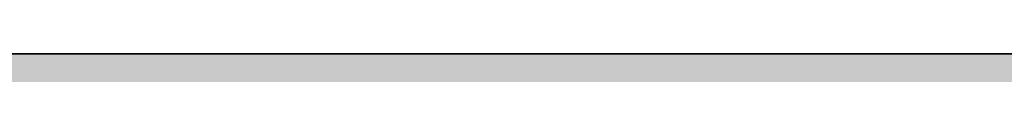
# Model space of a CAD drawing. Units: inches. Extents: x 2091 to 2899, y 967 to 2217.
# Tile 53 of 256: x 2212.15117 to 2212.16216, y 1099.91883 to 1099.91906. Entities that reach past the tile are written whole.
import ezdxf

# ---------------------------------------------------------------- set-up
doc = ezdxf.new("R2010")
doc.units = ezdxf.units.IN
doc.layers.add('A-WALL-PATT', color=141, linetype='Continuous', lineweight=13, true_color=0xadddf7)
doc.layers.add('L-SITE-WALL', color=7, linetype='Continuous', lineweight=35)

msp = doc.modelspace()

# ---------------------------------------------------------------- hatches: boundary and pattern name
at = {"layer": 'A-WALL-PATT'}
h = msp.add_hatch(color=256, dxfattribs=at)
h.dxf.hatch_style = 1
h.paths.add_polyline_path([(2212.143603, 1941.419059), (2387.643603, 1941.419059), (2387.643603, 1824.419059), (2392.143603, 1824.419059), (2392.143603, 1941.419059), (2609.643603, 1941.419059), (2609.643603, 1825.919059), (2614.143603, 1825.919059), (2614.143603, 1941.419059), (2794.143603, 1941.419059), (2794.143603, 1928.762166), (2803.143603, 1928.762166), (2803.143603, 2050.919059), (2203.143603, 2050.919059), (2203.143603, 1900.757859), (2212.143603, 1900.757859)])
h.paths.add_polyline_path([(2212.143603, 1945.919059), (2212.143603, 2041.919059), (2794.143603, 2041.919059), (2794.143603, 1945.919059), (2402.248245, 1945.919059), (2401.102434, 1945.775832), (2398.702434, 1945.775832)], flags=16)
h.paths.add_polyline_path([(2230.229861, 1948.062793), (2227.349861, 1949.502793), (2225.909861, 1951.902793), (2223.989861, 1952.862793), (2223.029861, 1955.262793), (2222.069861, 1959.582793), (2222.069861, 1963.422793), (2223.029861, 1965.662793), (2223.989861, 1965.342793), (2225.58591, 1963.860747), (2226.911533, 1964.957259), (2226.948861, 1965.938793), (2227.778319, 1966.952143), (2228.199916, 1968.878704), (2230.709861, 1964.862793), (2233.589861, 1966.302793), (2233.607309, 1966.331873), (2233.772659, 1964.938205), (2234.633802, 1963.676473), (2235.029861, 1963.902793), (2236.282035, 1965.572358), (2235.989861, 1962.942793), (2237.954512, 1957.540002), (2238.389861, 1957.902793), (2239.215861, 1960.305793), (2238.654565, 1966.38496), (2238.692792, 1966.438069), (2238.840578, 1967.499707), (2238.780291, 1967.687486), (2238.880538, 1967.786763), (2238.666861, 1966.251793), (2239.215861, 1960.305793), (2238.389861, 1957.902793), (2236.949861, 1956.702793), (2234.549861, 1949.982793)], flags=0)
h.paths.add_polyline_path([(2278.011974, 1948.062793), (2276.496427, 1947.873349), (2275.849833, 1947.688608), (2274.651974, 1947.102793)], flags=0)
h.paths.add_polyline_path([(2269.851974, 1955.742793), (2268.276176, 1956.629329), (2270.867302, 1956.348398), (2269.371974, 1958.142793), (2268.714964, 1959.192325), (2270.569833, 1958.728608), (2268.580725, 1961.906087), (2270.811974, 1960.891883), (2270.811974, 1963.422793), (2271.393315, 1964.779256), (2270.291762, 1966.156196), (2271.771974, 1965.662793), (2272.141387, 1966.524757), (2273.929833, 1965.928608), (2275.630385, 1968.054299), (2276.331938, 1966.72186), (2276.520431, 1966.952143), (2276.942029, 1968.878704), (2277.734293, 1967.611082), (2278.139888, 1969.46452), (2279.659124, 1967.033742), (2280.411974, 1966.782793), (2280.949302, 1967.588785), (2281.609833, 1967.368608), (2282.133266, 1968.153758), (2282.349235, 1966.333445), (2282.349849, 1966.332585), (2283.40755, 1968.09542), (2283.712631, 1965.52402), (2284.320221, 1964.633789), (2284.511809, 1964.889239), (2284.234974, 1965.704793), (2284.500472, 1967.318958), (2284.907944, 1965.41742), (2285.396313, 1966.068579), (2285.432833, 1966.290608), (2285.473338, 1966.171279), (2286.353919, 1967.345387), (2286.222007, 1966.158173), (2287.663492, 1968.080154), (2287.713974, 1968.442793), (2288.481599, 1969.016679), (2288.573993, 1968.728897), (2288.917461, 1969.06904), (2288.606833, 1966.837608), (2288.928726, 1963.35131), (2288.934974, 1963.356793), (2288.929731, 1963.340422), (2289.015281, 1962.413869), (2290.111223, 1963.875126), (2290.132833, 1963.942608), (2290.217672, 1964.017058), (2290.111223, 1963.875126), (2289.155833, 1960.891608), (2288.594036, 1959.257227), (2288.571974, 1959.102793), (2289.531974, 1960.542793), (2290.011974, 1962.462793), (2290.19184, 1962.642659), (2289.769833, 1959.688608), (2286.889833, 1957.288608), (2284.489833, 1950.568608), (2283.314658, 1950.046308), (2283.291974, 1949.982793), (2280.290059, 1948.648608), (2281.129833, 1948.648608), (2282.569833, 1948.168608), (2283.204726, 1948.062793), (2278.971974, 1948.062793), (2276.091974, 1949.502793), (2274.651974, 1951.902793), (2272.731974, 1952.862793)], flags=0)
h.paths.add_polyline_path([(2271.158868, 1958.021765), (2272.969833, 1955.848608), (2272.009833, 1960.168608), (2272.009833, 1964.008608), (2272.624426, 1965.442658), (2274.328023, 1963.860747), (2275.653646, 1964.957259), (2275.637743, 1964.53909), (2277.412231, 1966.006888), (2277.032974, 1965.156793), (2276.829924, 1964.975597), (2276.766012, 1963.295014), (2277.449635, 1962.66022), (2279.451974, 1964.862793), (2282.331974, 1966.302793), (2283.529833, 1966.888608), (2283.294512, 1966.770948), (2283.912993, 1963.8847), (2284.899249, 1964.448275), (2284.731974, 1962.942793), (2286.696625, 1957.540002), (2287.131974, 1957.902793), (2287.541913, 1959.095388), (2287.779395, 1958.442311), (2285.682738, 1956.695097), (2285.876503, 1959.795336), (2284.731974, 1962.942793), (2284.899249, 1964.448275), (2283.912993, 1963.8847), (2284.223833, 1962.434116), (2283.424365, 1963.605484), (2281.609833, 1962.568608), (2281.129833, 1960.168608), (2282.089833, 1956.328608), (2283.049833, 1952.968608), (2282.569833, 1950.568608), (2280.169833, 1948.648608), (2279.883316, 1948.791867), (2278.971974, 1948.062793), (2278.971974, 1949.022793), (2278.672313, 1949.397368), (2277.289833, 1950.088608), (2275.849833, 1952.488608), (2273.929833, 1953.448608), (2272.489833, 1954.888608), (2271.921647, 1954.888608), (2271.771974, 1955.262793)], flags=0)
h.paths.add_polyline_path([(2311.994146, 1955.742793), (2312.062717, 1955.674221), (2312.0551, 1955.7085)], flags=0)
h.paths.add_polyline_path([(2331.956146, 1963.951793), (2333.396146, 1965.391793), (2331.077146, 1963.356793), (2330.998603, 1963.111517)], flags=0)
h.paths.add_polyline_path([(2310.554146, 1954.302793), (2307.039807, 1956.279943), (2310.762903, 1955.876284), (2312.474146, 1953.822793), (2313.434146, 1951.422793), (2315.354146, 1950.462793), (2316.794146, 1948.062793), (2317.466146, 1947.726793), (2319.368691, 1947.964611), (2317.754146, 1949.982793), (2317.569531, 1950.610485), (2316.794146, 1951.902793), (2314.874146, 1952.862793), (2313.914146, 1955.262793), (2311.514146, 1958.142793), (2309.375489, 1961.559168), (2311.514146, 1960.337078), (2311.514146, 1961.982793), (2310.604672, 1963.119635), (2311.726605, 1962.47853), (2312.418332, 1964.09256), (2312.255964, 1964.29552), (2313.194146, 1963.982793), (2313.914146, 1965.662793), (2314.646778, 1965.418582), (2315.354146, 1966.302793), (2316.794146, 1967.742793), (2316.157435, 1966.946904), (2317.034111, 1965.28186), (2317.222604, 1965.512143), (2317.777048, 1968.045771), (2318.474111, 1966.72186), (2318.662604, 1966.952143), (2319.084201, 1968.878704), (2321.207049, 1965.482147), (2322.161419, 1966.913702), (2322.554146, 1966.782793), (2322.785988, 1967.130555), (2322.881646, 1966.324293), (2323.312041, 1965.72174), (2323.651289, 1965.891364), (2324.3965, 1967.133382), (2324.656945, 1964.938205), (2324.971986, 1964.476611), (2325.38728, 1967.001499), (2325.940813, 1964.418348), (2327.228929, 1966.135836), (2327.16632, 1965.572358), (2328.059139, 1966.762783), (2328.224576, 1966.247486), (2329.667971, 1967.67691), (2329.664576, 1967.687486), (2329.764823, 1967.786763), (2329.551146, 1966.251793), (2330.100146, 1960.305793), (2329.332814, 1958.07347), (2329.313065, 1957.935225), (2329.634146, 1958.202793), (2330.234146, 1959.102793), (2330.714146, 1961.022793), (2331.034146, 1961.342793), (2330.714146, 1959.102793), (2329.634146, 1958.202793), (2329.274146, 1957.662793), (2327.712112, 1956.361098), (2325.434146, 1949.982793), (2324.333769, 1949.493736), (2323.994146, 1948.542793), (2319.674146, 1946.622793), (2316.794146, 1948.062793), (2315.354146, 1950.462793), (2313.434146, 1951.422793)], flags=0)
h.paths.add_polyline_path([(2321.335684, 1947.952023), (2321.114146, 1948.062793), (2321.114146, 1949.022793), (2319.194146, 1951.422793), (2316.794146, 1959.582793), (2316.663237, 1959.582793), (2315.354146, 1958.142793), (2314.394146, 1958.142793), (2313.148303, 1958.709085), (2312.954146, 1959.582793), (2312.954146, 1960.891883), (2315.834146, 1959.582793), (2316.663237, 1959.582793), (2317.314709, 1960.299412), (2315.030195, 1962.420747), (2316.355818, 1963.517259), (2316.372337, 1963.951615), (2316.470195, 1963.860747), (2317.795818, 1964.957259), (2317.755219, 1963.889687), (2319.175146, 1965.156793), (2319.498407, 1965.881372), (2321.114146, 1965.342793), (2323.235885, 1962.372358), (2325.686349, 1963.772623), (2325.542789, 1962.480576), (2325.198783, 1963.494014), (2324.47851, 1963.082429), (2324.926005, 1960.994116), (2324.078087, 1962.236473), (2322.414791, 1961.286018), (2322.074146, 1959.582793), (2323.034146, 1955.742793), (2323.994146, 1952.382793), (2323.514146, 1949.982793), (2322.142717, 1948.88565), (2322.074146, 1948.542793)], flags=0)
h.paths.add_polyline_path([(2320.207479, 1963.337459), (2320.154146, 1963.422793), (2320.394146, 1963.542793)], flags=0)
h.paths.add_polyline_path([(2353.850527, 1965.8105), (2354.030527, 1965.7505), (2354.330527, 1966.4505), (2354.330527, 1966.9305)], flags=0)
h.paths.add_polyline_path([(2359.020582, 1969.026412), (2359.098382, 1968.901932), (2359.233527, 1969.5195), (2359.233527, 1969.9995)], flags=0)
h.paths.add_polyline_path([(2358.256694, 1966.681672), (2357.983601, 1966.348035), (2358.211267, 1966.146175), (2358.410492, 1966.389568)], flags=0)
h.paths.add_polyline_path([(2357.768473, 1966.058778), (2357.7322, 1965.104967), (2357.751047, 1965.120556), (2357.769527, 1965.6065), (2357.769527, 1966.057843)], flags=0)
h.paths.add_polyline_path([(2359.111527, 1965.3045), (2359.111527, 1964.8245), (2359.844527, 1966.4675), (2359.844527, 1966.9475)], flags=0)
h.paths.add_polyline_path([(2360.223684, 1966.621449), (2360.698527, 1969.3625), (2360.698527, 1969.8425), (2360.210527, 1967.0255), (2360.210527, 1966.6425)], flags=0)
h.paths.add_polyline_path([(2363.450527, 1967.8905), (2363.450527, 1968.3705), (2362.490527, 1966.9305), (2362.656045, 1966.698776)], flags=0)
h.paths.add_polyline_path([(2364.475523, 1966.078826), (2365.850527, 1968.3705), (2365.850527, 1968.8505), (2364.427975, 1966.479581)], flags=0)
h.paths.add_polyline_path([(2366.313527, 1965.8525), (2366.366709, 1965.695829), (2366.802527, 1968.3455), (2366.802527, 1968.8255)], flags=0)
h.paths.add_polyline_path([(2367.16531, 1965.803544), (2367.290527, 1966.9305), (2367.290527, 1967.4105), (2367.102701, 1965.720066)], flags=0)
h.paths.add_polyline_path([(2370.036527, 1959.9735), (2371.013527, 1963.0245), (2371.013527, 1963.5045), (2370.036527, 1960.4535)], flags=0)
h.paths.add_polyline_path([(2371.610527, 1960.2105), (2372.570527, 1961.6505), (2372.570527, 1962.1305), (2371.802527, 1960.9785)], flags=0)
h.paths.add_polyline_path([(2350.873666, 1956.005086), (2351.930527, 1955.8905), (2354.490527, 1953.3305), (2353.850527, 1954.9305), (2351.450527, 1957.8105), (2347.935527, 1963.4255), (2347.935527, 1963.9055), (2351.450527, 1958.2905), (2353.705073, 1955.585046), (2352.890527, 1959.2505), (2352.890527, 1959.7305), (2352.890527, 1961.924786), (2356.730527, 1959.7305), (2358.454471, 1961.626838), (2354.810527, 1965.0105), (2355.030855, 1965.28591), (2358.691091, 1961.88712), (2361.530527, 1965.0105), (2364.376495, 1966.433484), (2364.524394, 1965.186911), (2365.454468, 1963.824181), (2365.881073, 1964.067955), (2365.370527, 1966.4505), (2365.370527, 1966.9305), (2366.810527, 1960.2105), (2366.810527, 1959.7305), (2366.388709, 1952.981409), (2367.770527, 1956.8505), (2368.641225, 1957.576082), (2366.810527, 1962.6105), (2366.810527, 1963.0905), (2368.775179, 1957.68771), (2369.210527, 1958.0505), (2370.001592, 1960.351867), (2369.475232, 1966.052668), (2369.513458, 1966.105777), (2369.514173, 1966.110912), (2369.475232, 1966.532668), (2369.513458, 1966.585777), (2369.614635, 1967.312591), (2369.182527, 1968.6585), (2369.182527, 1969.1385), (2369.600957, 1967.835194), (2369.701204, 1967.934471), (2369.717947, 1968.054743), (2370.145176, 1968.374145), (2369.778707, 1968.011224), (2369.701204, 1967.454471), (2370.468161, 1968.214004), (2369.674936, 1967.265771), (2369.514173, 1966.110912), (2370.036527, 1960.4535), (2370.036527, 1959.9735), (2369.441756, 1958.243191), (2370.650527, 1959.2505), (2371.045821, 1962.017559), (2371.130527, 1962.1305), (2370.650527, 1958.7705), (2367.770527, 1956.3705), (2365.370527, 1949.6505), (2362.079099, 1948.187643), (2363.450527, 1947.7305), (2361.050527, 1947.7305), (2360.090527, 1947.7305), (2357.103861, 1947.357167), (2360.090527, 1948.2105), (2358.170527, 1949.1705), (2356.730527, 1951.5705), (2354.810527, 1952.5305), (2351.930527, 1955.4105)], flags=0)
h.paths.add_polyline_path([(2361.050527, 1948.6905), (2359.130527, 1951.0905), (2356.730527, 1959.2505), (2355.770527, 1959.2505), (2352.890527, 1960.559591), (2352.890527, 1961.444786), (2355.890527, 1959.7305), (2356.730527, 1959.7305), (2356.837194, 1959.367834), (2361.530527, 1964.5305), (2363.248422, 1965.389448), (2364.92531, 1963.041805), (2362.490527, 1961.6505), (2362.063861, 1959.517167), (2362.970527, 1955.8905), (2363.930527, 1952.5305), (2363.930527, 1952.0505), (2363.450527, 1949.6505), (2361.050527, 1947.7305)], flags=0)
h.paths.add_polyline_path([(2359.130527, 1951.5705), (2359.290527, 1951.3705), (2361.050527, 1954.4505), (2361.050527, 1954.9305)], flags=0)
h.paths.add_polyline_path([(2357.219527, 1966.5455), (2356.792527, 1968.8145), (2356.792527, 1969.2945), (2357.219527, 1967.0255)], flags=0)
h.paths.add_polyline_path([(2361.050527, 1954.4505), (2361.530527, 1958.7705), (2361.530527, 1959.2505), (2361.050527, 1954.9305)], flags=0)
h.paths.add_polyline_path([(2402.548287, 1948.486076), (2402.302434, 1948.415832), (2402.590434, 1948.415832)], flags=0)
h.paths.add_polyline_path([(2394.142434, 1956.095832), (2395.685052, 1954.553214), (2396.720495, 1953.970679), (2396.062434, 1955.615832), (2395.241381, 1956.601096), (2395.878904, 1956.441715), (2395.102434, 1959.935832), (2395.102434, 1963.775832), (2396.062434, 1966.015832), (2397.022434, 1965.695832), (2398.618483, 1964.213787), (2399.944106, 1965.310299), (2399.981434, 1966.291832), (2400.810891, 1967.305183), (2401.232489, 1969.231744), (2403.537949, 1965.543008), (2403.941984, 1967.389316), (2404.702434, 1967.135832), (2405.460328, 1966.07478), (2406.622434, 1966.655832), (2406.639882, 1966.684913), (2406.805232, 1965.291245), (2406.925694, 1965.114746), (2407.342434, 1964.975832), (2407.874326, 1965.77367), (2408.1691, 1964.398055), (2409.314608, 1965.925398), (2409.217458, 1965.051054), (2409.445232, 1963.131245), (2410.306374, 1961.869513), (2410.702434, 1962.095832), (2411.442269, 1963.082279), (2411.165434, 1963.897832), (2411.616426, 1966.639757), (2411.725365, 1966.791109), (2411.873151, 1967.852747), (2411.812864, 1968.040526), (2411.913111, 1968.139803), (2411.699434, 1966.604832), (2412.248434, 1960.658832), (2413.225434, 1963.709832), (2414.3779, 1964.72116), (2414.513151, 1965.692747), (2414.452864, 1965.880526), (2414.553111, 1965.979803), (2414.3779, 1964.72116), (2414.519817, 1964.845697), (2414.365365, 1964.631109), (2414.339434, 1964.444832), (2414.888434, 1958.498832), (2414.062434, 1956.095832), (2412.622434, 1954.895832), (2410.17137, 1948.032854), (2410.016719, 1948.084404), (2405.902434, 1946.255832), (2405.902434, 1947.215832), (2405.204252, 1948.08856), (2404.222434, 1948.415832), (2403.262434, 1948.415832), (2400.382434, 1949.855832), (2399.662434, 1951.055832), (2397.982434, 1952.735832), (2397.022434, 1953.215832), (2395.685052, 1954.553214), (2392.656776, 1956.256908)], flags=0)
h.paths.add_polyline_path([(2409.08565, 1964.407441), (2409.130363, 1964.275715), (2409.262434, 1964.495832)], flags=0)
h.paths.add_polyline_path([(2397.742434, 1961.615832), (2398.702434, 1963.855832), (2399.662434, 1963.535832), (2401.426563, 1965.740994), (2401.791415, 1966.5588), (2402.071434, 1965.070832), (2402.835507, 1964.393367), (2403.262398, 1964.9149), (2403.338119, 1964.771086), (2402.615516, 1963.976223), (2402.498612, 1960.902238), (2403.542997, 1959.932452), (2404.413203, 1960.889679), (2404.702434, 1962.335832), (2407.916347, 1964.172354), (2409.520211, 1961.926944), (2410.987085, 1957.893042), (2411.422434, 1958.255832), (2412.047964, 1960.075625), (2412.410341, 1959.079088), (2411.675621, 1958.466821), (2411.662434, 1958.255832), (2411.62607, 1958.425529), (2409.982434, 1957.055832), (2407.582434, 1950.335832), (2403.262434, 1948.415832), (2403.262434, 1949.375832), (2401.342434, 1951.775832), (2399.416508, 1958.323981), (2397.742434, 1959.084923), (2397.742434, 1959.970118), (2397.102434, 1960.335832), (2397.742434, 1960.044923)], flags=0)
h.paths.add_polyline_path([(2405.902434, 1952.975832), (2405.950434, 1953.407832), (2406.016719, 1953.175832)], flags=0)
h.paths.add_polyline_path([(2449.817778, 1967.114014), (2449.752323, 1967.135832), (2449.793703, 1967.077901)], flags=0)
h.paths.add_polyline_path([(2451.697696, 1966.61812), (2451.740895, 1966.690118), (2451.692051, 1966.665696)], flags=0)
h.paths.add_polyline_path([(2454.343628, 1965.737572), (2455.752323, 1967.615832), (2455.992323, 1968.095832), (2454.364497, 1965.925398)], flags=0)
h.paths.add_polyline_path([(2457.547323, 1968.863832), (2457.787323, 1969.343832), (2457.054323, 1968.795832), (2457.007622, 1968.460345)], flags=0)
h.paths.add_polyline_path([(2456.921784, 1967.856662), (2456.802238, 1968.229016), (2456.723, 1967.659803)], flags=0)
h.paths.add_polyline_path([(2457.302323, 1967.376832), (2457.542323, 1967.856832), (2456.810323, 1966.839832), (2456.740516, 1966.700218), (2456.749021, 1966.608105)], flags=0)
h.paths.add_polyline_path([(2458.275323, 1963.709832), (2458.155343, 1963.335153), (2460.354323, 1965.264832), (2460.594323, 1965.744832)], flags=0)
h.paths.add_polyline_path([(2458.392323, 1962.815832), (2458.364088, 1962.618185), (2459.592323, 1964.255832), (2459.832323, 1964.735832)], flags=0)
h.paths.add_polyline_path([(2459.352323, 1962.815832), (2459.272323, 1962.495832), (2460.072323, 1963.295832), (2460.312323, 1963.775832)], flags=0)
h.paths.add_polyline_path([(2458.680323, 1960.607832), (2458.632323, 1960.415832), (2459.592323, 1961.855832), (2459.832323, 1962.335832)], flags=0)
h.paths.add_polyline_path([(2437.83817, 1956.24265), (2439.192323, 1956.095832), (2441.352323, 1953.935832), (2440.872323, 1955.135832), (2438.472323, 1958.015832), (2438.071563, 1958.656023), (2438.712323, 1958.495832), (2440.639596, 1956.183105), (2439.912323, 1959.455832), (2439.912323, 1963.295832), (2441.352323, 1966.655832), (2441.592323, 1967.135832), (2441.112323, 1966.015832), (2442.072323, 1965.695832), (2443.988993, 1968.09167), (2444.241323, 1966.750832), (2444.916801, 1966.15192), (2445.676574, 1967.080136), (2446.255323, 1969.724832), (2446.495323, 1970.204832), (2446.282379, 1969.231744), (2447.362672, 1967.503275), (2447.720323, 1969.567832), (2447.960323, 1970.047832), (2447.48548, 1967.306781), (2448.792323, 1965.215832), (2448.472323, 1964.863832), (2448.552323, 1964.735832), (2451.452051, 1966.185696), (2451.615122, 1964.811245), (2452.307917, 1963.796172), (2453.234505, 1964.325651), (2454.072323, 1960.415832), (2453.628687, 1953.317651), (2454.792323, 1956.575832), (2455.032323, 1957.055832), (2455.718835, 1957.627926), (2453.832323, 1962.815832), (2453.940966, 1963.793615), (2453.335323, 1965.577832), (2453.824323, 1968.550832), (2454.064323, 1969.030832), (2453.575323, 1966.057832), (2454.040333, 1964.687919), (2453.832323, 1962.815832), (2455.718835, 1957.627926), (2456.367207, 1958.168235), (2457.058323, 1960.178832), (2457.298323, 1960.658832), (2456.472323, 1958.255832), (2457.717729, 1959.29367), (2457.672323, 1958.975832), (2454.889951, 1956.657188), (2453.614142, 1953.084923), (2453.592323, 1952.735832), (2453.352323, 1952.255832), (2453.359596, 1952.372196), (2452.632323, 1950.335832), (2452.392323, 1949.855832), (2449.203752, 1948.43869), (2450.712323, 1947.935832), (2448.072323, 1947.935832), (2447.112323, 1947.935832), (2444.552323, 1947.615832), (2447.199596, 1948.372196), (2445.192323, 1949.375832), (2443.752323, 1951.775832), (2441.832323, 1952.735832), (2438.952323, 1955.615832)], flags=0)
h.paths.add_polyline_path([(2443.992323, 1959.935832), (2444.040323, 1959.772632), (2444.121554, 1959.861986)], flags=0)
h.paths.add_polyline_path([(2442.912323, 1959.935832), (2443.032323, 1959.935832), (2442.445657, 1960.202499)], flags=0)
h.paths.add_polyline_path([(2444.982943, 1965.019677), (2445.279323, 1965.264832), (2445.519323, 1965.744832), (2444.993996, 1965.310299)], flags=0)
h.paths.add_polyline_path([(2446.133323, 1965.029832), (2446.330366, 1965.471499), (2444.970323, 1964.257832), (2444.730323, 1963.777832)], flags=0)
h.paths.add_polyline_path([(2442.792323, 1959.455832), (2443.752323, 1959.455832), (2446.152323, 1951.295832), (2446.412323, 1951.750832), (2446.392323, 1951.775832), (2448.080599, 1954.730315), (2448.552323, 1958.975832), (2441.832323, 1965.215832), (2442.154946, 1965.619111), (2448.792323, 1959.455832), (2448.312323, 1955.135832), (2448.072323, 1954.655832), (2446.412323, 1951.750832), (2448.312323, 1949.375832), (2448.312323, 1948.415832), (2450.540895, 1950.19869), (2450.952323, 1952.255832), (2449.992323, 1955.615832), (2449.032323, 1959.455832), (2449.512323, 1961.855832), (2449.752323, 1962.335832), (2449.674904, 1961.948736), (2452.994505, 1963.845651), (2453.064414, 1963.519409), (2452.884611, 1963.782854), (2449.674904, 1961.948736), (2449.272323, 1959.935832), (2450.232323, 1956.095832), (2451.192323, 1952.735832), (2450.712323, 1950.335832), (2450.472323, 1949.855832), (2448.072323, 1947.935832), (2448.072323, 1948.535832), (2445.432323, 1949.855832), (2443.992323, 1952.255832), (2442.072323, 1953.215832), (2441.112323, 1955.615832), (2440.152323, 1959.935832), (2440.152323, 1960.655832)], flags=0)
h.paths.add_polyline_path([(2456.692323, 1966.985832), (2457.608323, 1968.080832), (2457.848323, 1968.560832), (2456.932323, 1967.465832)], flags=0)
h.paths.add_polyline_path([(2489.89657, 1966.580241), (2489.942948, 1966.189347), (2490.747488, 1967.530248), (2491.319122, 1968.951161)], flags=0)
h.paths.add_polyline_path([(2473.562471, 1956.407131), (2477.139981, 1956.019257), (2476.955333, 1956.240834), (2475.108049, 1957.280108), (2476.347488, 1956.970248), (2475.186901, 1958.824216), (2476.919122, 1958.391161), (2475.411642, 1960.799269), (2477.787488, 1959.719339), (2477.787488, 1962.250248), (2477.637399, 1962.43786), (2477.82255, 1962.332059), (2478.359122, 1963.58406), (2478.359122, 1963.671161), (2477.324348, 1964.964628), (2478.714826, 1964.501135), (2479.319122, 1965.911161), (2480.279122, 1965.591161), (2481.783965, 1967.472214), (2482.116488, 1965.705248), (2482.880562, 1965.027782), (2483.209305, 1965.429408), (2483.220169, 1965.71509), (2483.07594, 1965.989022), (2483.711762, 1966.765808), (2484.130488, 1968.679248), (2484.702122, 1970.100161), (2484.489177, 1969.127072), (2486.502904, 1965.905109), (2487.387488, 1965.610248), (2488.153419, 1966.759144), (2488.717017, 1965.970108), (2489.200086, 1966.211642), (2489.330671, 1965.110992), (2490.393905, 1963.622465), (2490.660765, 1963.774956), (2490.493905, 1964.553636), (2490.923063, 1963.924841), (2491.319122, 1964.151161), (2491.333389, 1964.170183), (2491.210488, 1964.532248), (2491.281756, 1964.965537), (2491.425789, 1964.293383), (2494.076476, 1967.827632), (2494.497918, 1966.514942), (2494.598165, 1966.614218), (2494.689488, 1967.270248), (2495.106748, 1967.582196), (2495.129839, 1967.748075), (2495.069552, 1967.935854), (2495.169799, 1968.035131), (2495.031777, 1967.043632), (2495.753818, 1967.758684), (2494.982053, 1966.686437), (2494.956122, 1966.500161), (2495.479021, 1960.836851), (2495.910488, 1962.184248), (2496.482122, 1963.605161), (2496.072694, 1962.326589), (2496.768904, 1962.937536), (2496.599122, 1962.711161), (2496.119122, 1959.351161), (2496.732873, 1960.271787), (2496.987488, 1961.290248), (2497.559122, 1962.711161), (2497.079122, 1960.791161), (2496.507488, 1959.370248), (2495.547488, 1957.930248), (2492.758842, 1955.606376), (2490.839122, 1950.231161), (2490.267488, 1948.810248), (2485.947488, 1946.890248), (2483.067488, 1948.330248), (2481.627488, 1950.730248), (2479.707488, 1951.690248), (2476.827488, 1954.570248)], flags=0)
h.paths.add_polyline_path([(2485.576973, 1948.313392), (2485.559122, 1948.311161), (2485.578758, 1948.311161)], flags=0)
h.paths.add_polyline_path([(2478.645063, 1954.551161), (2478.109042, 1956.963257), (2479.319122, 1955.511161), (2480.279122, 1953.111161), (2482.199122, 1952.151161), (2483.639122, 1949.751161), (2486.519122, 1948.311161), (2486.519122, 1949.271161), (2484.739307, 1951.49593), (2484.027488, 1950.250248), (2481.627488, 1958.410248), (2482.375148, 1959.232673), (2482.199122, 1959.831161), (2483.197572, 1960.929456), (2479.707488, 1964.170248), (2480.603358, 1965.290085), (2481.875171, 1964.109115), (2482.666387, 1964.763582), (2482.615359, 1963.421798), (2482.989199, 1963.074661), (2484.008488, 1963.984248), (2484.683606, 1965.497507), (2484.580122, 1965.405161), (2485.357268, 1967.147113), (2485.120645, 1965.781197), (2486.427488, 1963.690248), (2488.145383, 1964.549195), (2489.822271, 1962.201552), (2490.747488, 1962.730248), (2491.999662, 1964.399813), (2492.076046, 1965.087265), (2492.212892, 1964.684119), (2492.485374, 1965.047429), (2492.279122, 1963.191161), (2494.243773, 1957.78837), (2494.562503, 1958.053978), (2494.933488, 1959.133248), (2495.505122, 1960.554161), (2494.679122, 1958.151161), (2494.107488, 1956.730248), (2494.562503, 1958.053978), (2493.408544, 1957.092345), (2491.707488, 1961.770248), (2491.999662, 1964.399813), (2490.747488, 1962.730248), (2487.71203, 1960.9957), (2487.479122, 1959.831161), (2488.439122, 1955.991161), (2489.399122, 1952.631161), (2488.919122, 1950.231161), (2488.576918, 1949.957397), (2488.347488, 1948.810248), (2487.651715, 1948.253629), (2487.479122, 1948.311161), (2486.519122, 1948.311161), (2483.639122, 1949.751161), (2482.199122, 1952.151161), (2480.279122, 1953.111161), (2478.839122, 1954.551161)], flags=0)
h.paths.add_polyline_path([(2526.648252, 1966.987524), (2526.517343, 1967.031161), (2526.600102, 1966.915298)], flags=0)
h.paths.add_polyline_path([(2528.47064, 1966.446656), (2528.574486, 1966.619732), (2528.457071, 1966.561025)], flags=0)
h.paths.add_polyline_path([(2534.133343, 1967.496161), (2534.156685, 1967.542845), (2534.059841, 1967.408296)], flags=0)
h.paths.add_polyline_path([(2536.161923, 1964.0506), (2535.157343, 1962.711161), (2535.100872, 1962.315866), (2536.117343, 1963.671161), (2536.420532, 1964.277539)], flags=0)
h.paths.add_polyline_path([(2535.157343, 1959.831161), (2536.117343, 1961.271161), (2536.597343, 1962.231161), (2535.253343, 1960.215161)], flags=0)
h.paths.add_polyline_path([(2513.249035, 1956.284796), (2516.221181, 1955.962555), (2514.997343, 1957.431161), (2514.195823, 1958.711541), (2515.477343, 1958.391161), (2516.931888, 1956.645706), (2516.437343, 1958.871161), (2516.437343, 1962.711161), (2516.872692, 1963.726974), (2515.346434, 1965.634797), (2517.397343, 1964.951161), (2517.877343, 1966.071161), (2518.357343, 1967.031161), (2517.877343, 1965.911161), (2518.837343, 1965.591161), (2520.48659, 1967.652719), (2520.766343, 1966.166161), (2521.530417, 1965.488695), (2521.781443, 1965.795375), (2521.800911, 1966.307268), (2521.477804, 1966.920936), (2521.246343, 1967.126161), (2521.177701, 1967.490913), (2521.477804, 1966.920936), (2522.010417, 1966.448695), (2522.257386, 1966.750417), (2522.780343, 1969.140161), (2523.260343, 1970.100161), (2523.047398, 1969.127072), (2524.673132, 1966.525897), (2526.037343, 1966.071161), (2526.795238, 1965.010108), (2527.977071, 1965.601025), (2528.140141, 1964.226573), (2528.66459, 1963.458159), (2529.388616, 1963.871888), (2529.329665, 1964.14699), (2529.481284, 1963.924841), (2529.877343, 1964.151161), (2529.98401, 1964.293383), (2529.789053, 1965.20318), (2530.0624, 1964.397903), (2532.802483, 1968.051347), (2533.147773, 1966.975854), (2533.24802, 1967.075131), (2533.339343, 1967.731161), (2533.672848, 1967.980493), (2533.72802, 1968.035131), (2533.514343, 1966.500161), (2534.024718, 1960.972496), (2534.560343, 1962.645161), (2535.040343, 1963.605161), (2534.063343, 1960.554161), (2533.237343, 1958.151161), (2534.288154, 1959.026836), (2534.197343, 1958.391161), (2531.512597, 1956.153872), (2529.397343, 1950.231161), (2528.917343, 1949.271161), (2526.448772, 1948.174018), (2527.477343, 1947.831161), (2530.357343, 1947.351161), (2524.597343, 1947.351161), (2521.717343, 1948.791161), (2520.277343, 1951.191161), (2518.357343, 1952.151161), (2515.477343, 1955.031161)], flags=0)
h.paths.add_polyline_path([(2523.93476, 1967.190308), (2523.619512, 1966.483689), (2523.7705, 1966.242109)], flags=0)
h.paths.add_polyline_path([(2518.837343, 1953.111161), (2517.877343, 1955.511161), (2516.884983, 1959.976779), (2516.917343, 1959.96207), (2516.917343, 1962.025446), (2520.757343, 1959.831161), (2522.024949, 1961.225527), (2518.357343, 1964.631161), (2519.002589, 1965.437718), (2520.433392, 1964.109115), (2521.30112, 1964.826871), (2521.245157, 1963.355333), (2525.638307, 1959.27598), (2526.037343, 1961.271161), (2529.397343, 1963.191161), (2530.649517, 1964.860726), (2530.66472, 1964.99755), (2530.691956, 1964.917311), (2531.087778, 1965.445074), (2530.945985, 1964.168944), (2530.691956, 1964.917311), (2529.397343, 1963.191161), (2526.362504, 1961.456967), (2526.037343, 1959.831161), (2526.997343, 1955.991161), (2527.957343, 1952.631161), (2527.477343, 1950.231161), (2527.134486, 1949.956875), (2526.973928, 1949.154087), (2526.697343, 1949.031161), (2524.597343, 1947.351161), (2524.597343, 1948.311161), (2524.277343, 1948.711161), (2522.197343, 1949.751161), (2520.757343, 1952.151161)], flags=0)
h.paths.add_polyline_path([(2520.277343, 1958.871161), (2520.853343, 1959.504761), (2523.157343, 1951.671161), (2524.613895, 1954.220126), (2524.597343, 1954.071161), (2522.677343, 1950.711161)], flags=0)
h.paths.add_polyline_path([(2559.37091, 1966.311161), (2559.398411, 1966.324911), (2559.401943, 1966.345296)], flags=0)
h.paths.add_polyline_path([(2549.77091, 1957.191161), (2552.65091, 1954.311161), (2552.133987, 1955.603468), (2550.61091, 1957.431161), (2547.09591, 1963.046161), (2545.77591, 1965.206161), (2549.29091, 1959.591161), (2551.69091, 1956.711161), (2550.792933, 1960.752059), (2550.73091, 1960.780251), (2550.73091, 1964.871161), (2551.69091, 1967.111161), (2552.65091, 1966.791161), (2554.246959, 1965.309115), (2555.034252, 1965.960337), (2555.581671, 1966.644612), (2555.60991, 1967.387161), (2556.439368, 1968.400511), (2556.860966, 1970.327072), (2559.37091, 1966.311161), (2560.69091, 1964.151161), (2562.408805, 1965.010108), (2561.65091, 1966.071161), (2560.33091, 1968.231161), (2561.758497, 1966.23254), (2562.347213, 1967.115614), (2562.433709, 1966.386573), (2563.127798, 1965.369604), (2563.57091, 1965.591161), (2563.588359, 1965.620241), (2563.362543, 1967.52354), (2563.722489, 1965.843792), (2565.060001, 1968.072979), (2564.732862, 1965.128722), (2565.117577, 1963.333383), (2567.444622, 1966.436109), (2567.315615, 1967.833328), (2567.353841, 1967.886437), (2567.501627, 1968.948075), (2567.44134, 1969.135854), (2567.541587, 1969.235131), (2567.32791, 1967.700161), (2567.87691, 1961.754161), (2568.746689, 1964.470327), (2568.635615, 1965.673328), (2568.673841, 1965.726437), (2568.821627, 1966.788075), (2568.76134, 1966.975854), (2568.861587, 1967.075131), (2568.64791, 1965.540161), (2568.726127, 1964.693026), (2568.85391, 1964.805161), (2568.746689, 1964.470327), (2568.817236, 1963.706261), (2568.97091, 1963.911161), (2568.866075, 1963.17731), (2569.19691, 1959.594161), (2568.37091, 1957.191161), (2566.93091, 1955.991161), (2564.620272, 1949.521373), (2564.65091, 1949.511161), (2564.616625, 1949.511161), (2564.53091, 1949.271161), (2560.21091, 1947.351161), (2557.33091, 1948.791161), (2556.045196, 1950.934018), (2556.01091, 1950.951161), (2555.856625, 1951.208303), (2553.97091, 1952.151161), (2551.09091, 1955.031161), (2546.650144, 1957.529515)], flags=0)
h.paths.add_polyline_path([(2567.025794, 1959.33023), (2567.035007, 1959.304895), (2567.05091, 1959.351161)], flags=0)
h.paths.add_polyline_path([(2551.968287, 1962.518374), (2553.01091, 1964.951161), (2553.97091, 1964.631161), (2555.566959, 1963.149115), (2556.892583, 1964.245627), (2556.92991, 1965.227161), (2557.143984, 1965.488695), (2556.420066, 1966.130557), (2556.391421, 1966.104995), (2556.37991, 1966.166161), (2556.420066, 1966.130557), (2556.95191, 1966.605161), (2557.092139, 1966.919478), (2557.570875, 1966.010228), (2557.759368, 1966.240511), (2557.41791, 1964.680161), (2556.892583, 1964.245627), (2556.807089, 1961.997566), (2560.69091, 1958.391161), (2560.635526, 1957.892699), (2560.81091, 1957.191161), (2561.77091, 1953.831161), (2561.29091, 1951.431161), (2559.110423, 1949.68677), (2559.156484, 1949.629193), (2563.02652, 1951.349209), (2562.61091, 1949.271161), (2560.21091, 1947.351161), (2560.21091, 1948.311161), (2559.25091, 1949.511161), (2558.89091, 1949.511161), (2558.89091, 1949.961161), (2558.29091, 1950.711161), (2558.053701, 1951.517672), (2556.97091, 1952.871161), (2555.06788, 1959.341464), (2552.05091, 1961.065446), (2552.05091, 1962.471161)], flags=0)
h.paths.add_polyline_path([(2588.330049, 1958.391161), (2588.610248, 1958.110962), (2588.553362, 1958.366949)], flags=0)
h.paths.add_polyline_path([(2594.745454, 1950.493086), (2593.957532, 1953.172022), (2593.130049, 1954.551161), (2591.210049, 1955.511161), (2590.250049, 1957.911161), (2588.309033, 1960.240379), (2586.177306, 1961.209346), (2587.850049, 1960.791161), (2587.253416, 1961.744246), (2588.441314, 1961.065446), (2588.441314, 1962.655528), (2588.421679, 1962.665345), (2588.441314, 1962.711161), (2586.914038, 1964.620256), (2588.877086, 1963.727962), (2589.290049, 1964.69154), (2589.290049, 1966.071161), (2590.250049, 1968.311161), (2591.210049, 1967.991161), (2592.806098, 1966.509115), (2594.131721, 1967.605627), (2594.169049, 1968.587161), (2594.998506, 1969.600511), (2595.420104, 1971.527072), (2597.930049, 1967.511161), (2600.810049, 1968.951161), (2600.827497, 1968.980241), (2600.992847, 1967.586573), (2601.853989, 1966.324841), (2602.107143, 1966.4695), (2602.236354, 1967.255069), (2602.356715, 1966.693383), (2603.502223, 1968.220726), (2603.210049, 1965.591161), (2605.1747, 1960.18837), (2605.506891, 1960.465196), (2605.026019, 1965.673328), (2605.064245, 1965.726437), (2605.212031, 1966.788075), (2605.151744, 1966.975854), (2605.251991, 1967.075131), (2605.343314, 1967.731161), (2605.952905, 1968.186898), (2605.874753, 1969.033328), (2605.912979, 1969.086437), (2606.060766, 1970.148075), (2606.000479, 1970.335854), (2606.100725, 1970.435131), (2605.887049, 1968.900161), (2606.436049, 1962.954161), (2605.610049, 1960.551161), (2605.997036, 1960.87365), (2606.564314, 1962.645161), (2608.241494, 1964.116941), (2608.010049, 1963.191161), (2607.050049, 1961.751161), (2606.631486, 1961.402358), (2606.201314, 1958.391161), (2603.321314, 1955.991161), (2600.921314, 1949.271161), (2596.601314, 1947.351161), (2593.721314, 1948.791161), (2592.857314, 1950.231161), (2592.650049, 1950.231161)], flags=0)
h.paths.add_polyline_path([(2596.601314, 1947.351161), (2596.601314, 1948.311161), (2594.681314, 1950.711161), (2596.154954, 1953.290029), (2595.530049, 1954.071161), (2593.199226, 1961.995957), (2592.65134, 1962.504708), (2591.780151, 1963.002531), (2593.282987, 1964.245627), (2593.320314, 1965.227161), (2594.149772, 1966.240511), (2594.57137, 1968.167072), (2596.182651, 1965.589023), (2596.951273, 1966.434508), (2598.041314, 1966.071161), (2598.799209, 1965.010108), (2599.961314, 1965.591161), (2599.978763, 1965.620241), (2600.144113, 1964.226573), (2601.005255, 1962.964841), (2601.401314, 1963.191161), (2602.653488, 1964.860726), (2602.361314, 1962.231161), (2603.792748, 1958.294719), (2601.977644, 1953.212427), (2601.946208, 1952.709453), (2599.468755, 1951.608363), (2599.001314, 1949.271161)], flags=0)
h.paths.add_polyline_path([(2597.561314, 1958.871161), (2597.670966, 1959.419419), (2597.595054, 1958.736204)], flags=0)
h.paths.add_polyline_path([(2623.666305, 1961.254375), (2625.519163, 1960.791161), (2624.965544, 1961.675533), (2627.199163, 1960.660251), (2627.199163, 1961.151161), (2626.959163, 1962.231161), (2626.959163, 1963.491161), (2625.582321, 1965.212213), (2626.959163, 1964.425446), (2626.959163, 1965.831161), (2626.869163, 1965.861161), (2627.919163, 1968.311161), (2628.879163, 1967.991161), (2630.475212, 1966.509115), (2631.800835, 1967.605627), (2631.838163, 1968.587161), (2632.667621, 1969.600511), (2633.089218, 1971.527072), (2635.599163, 1967.511161), (2638.479163, 1968.951161), (2638.496611, 1968.980241), (2638.661961, 1967.586573), (2639.176273, 1966.833011), (2639.780216, 1967.839582), (2640.02583, 1966.693383), (2641.171337, 1968.220726), (2640.879163, 1965.591161), (2641.114265, 1964.94463), (2641.411337, 1965.340726), (2641.308099, 1964.411586), (2642.843814, 1960.18837), (2643.279163, 1960.551161), (2644.084736, 1962.894736), (2643.783867, 1966.153328), (2643.806834, 1966.185237), (2643.600676, 1968.418053), (2643.522812, 1968.660581), (2643.72988, 1970.148075), (2643.669593, 1970.335854), (2643.76984, 1970.435131), (2643.556163, 1968.900161), (2643.600676, 1968.418053), (2643.909593, 1967.455854), (2644.00984, 1967.555131), (2643.811743, 1966.132079), (2644.105163, 1962.954161), (2644.238773, 1961.350836), (2644.719163, 1961.751161), (2645.032853, 1962.221695), (2645.322163, 1963.125161), (2646.07642, 1963.787047), (2645.032853, 1962.221695), (2644.345163, 1960.074161), (2643.519163, 1957.671161), (2642.079163, 1956.471161), (2639.719612, 1949.864419), (2639.875527, 1949.838433), (2635.359163, 1947.831161), (2632.479163, 1949.271161), (2631.039163, 1951.671161), (2629.119163, 1952.631161), (2628.159163, 1955.031161), (2625.759163, 1957.911161)], flags=0)
h.paths.add_polyline_path([(2627.816306, 1956.574018), (2627.373708, 1958.565706), (2626.376306, 1959.762589), (2627.199163, 1959.351161), (2627.373708, 1958.565706), (2627.919163, 1957.911161), (2628.879163, 1955.511161), (2630.799163, 1954.551161), (2632.239163, 1952.151161), (2633.315025, 1951.613229), (2631.039163, 1959.351161), (2631.49783, 1959.855694), (2630.799163, 1962.231161), (2631.449867, 1962.946935), (2630.715212, 1963.629115), (2632.040835, 1964.725627), (2632.078163, 1965.707161), (2632.292237, 1965.968695), (2631.705339, 1966.489067), (2633.136441, 1967.766144), (2633.329218, 1968.647072), (2634.674718, 1966.494272), (2635.208465, 1967.081393), (2636.799163, 1966.551161), (2637.676404, 1967.867023), (2638.993946, 1966.022465), (2639.705345, 1966.428979), (2641.119163, 1959.831161), (2640.930072, 1956.805706), (2639.439163, 1952.631161), (2638.227456, 1952.092624), (2637.759163, 1949.751161), (2635.359163, 1947.831161), (2635.359163, 1948.791161), (2633.439163, 1951.191161), (2633.315025, 1951.613229), (2632.239163, 1952.151161), (2630.799163, 1954.551161), (2628.879163, 1955.511161)], flags=0)
h.paths.add_polyline_path([(2637.759163, 1953.831161), (2637.279163, 1955.511161), (2636.319163, 1959.351161), (2636.799163, 1961.751161), (2639.233946, 1963.142465), (2637.557058, 1965.490108), (2638.738891, 1966.081025), (2638.901961, 1964.706573), (2639.763104, 1963.444841), (2636.799163, 1961.751161), (2636.532496, 1960.417827), (2637.039163, 1958.391161), (2637.999163, 1955.031161)], flags=0)
h.paths.add_polyline_path([(2668.567407, 1951.431161), (2667.607407, 1953.831161), (2665.207407, 1956.711161), (2662.293903, 1961.365307), (2665.447407, 1959.591161), (2666.647407, 1958.391161), (2666.647407, 1959.975161), (2666.058317, 1960.68207), (2666.647407, 1960.345446), (2666.647407, 1961.991161), (2666.70009, 1962.114087), (2666.407407, 1963.431161), (2666.407407, 1967.271161), (2667.367407, 1969.511161), (2668.327407, 1969.191161), (2669.923457, 1967.709115), (2671.24908, 1968.805627), (2671.286407, 1969.787161), (2672.115865, 1970.800511), (2672.537463, 1972.727072), (2675.047407, 1968.711161), (2677.927407, 1970.151161), (2677.944856, 1970.180241), (2678.110206, 1968.786573), (2678.971348, 1967.524841), (2679.367407, 1967.751161), (2680.619581, 1969.420726), (2680.327407, 1966.791161), (2682.292059, 1961.38837), (2682.727407, 1961.751161), (2683.358306, 1963.586571), (2683.232112, 1964.953328), (2683.270338, 1965.006437), (2683.393215, 1965.889138), (2683.359969, 1966.249215), (2683.357837, 1966.255854), (2683.359229, 1966.257232), (2682.992112, 1970.233328), (2683.030338, 1970.286437), (2683.178124, 1971.348075), (2683.117837, 1971.535854), (2683.218084, 1971.635131), (2683.004407, 1970.100161), (2683.359229, 1966.257232), (2683.458084, 1966.355131), (2683.393215, 1965.889138), (2683.413908, 1965.665023), (2684.42381, 1966.872275), (2683.553407, 1964.154161), (2683.358306, 1963.586571), (2683.793407, 1958.874161), (2682.967407, 1956.471161), (2681.527407, 1955.271161), (2680.109226, 1951.300251), (2680.084933, 1950.911573), (2679.976846, 1950.929587), (2679.127407, 1948.551161), (2674.807407, 1946.631161), (2671.927407, 1948.071161), (2670.487407, 1950.471161)], flags=0)
h.paths.add_polyline_path([(2671.935683, 1953.227023), (2671.687407, 1953.351161), (2670.247407, 1955.751161), (2668.327407, 1956.711161), (2667.356741, 1959.137827), (2669.527407, 1958.151161), (2670.487407, 1958.151161), (2671.479407, 1959.242361), (2670.684402, 1961.94538), (2668.889599, 1963.611982), (2667.307407, 1964.331161), (2668.567407, 1963.911161), (2668.830937, 1964.240572), (2670.247407, 1963.431161), (2672.42214, 1965.823367), (2672.777463, 1967.447072), (2673.234074, 1966.716494), (2674.411919, 1968.012124), (2673.980564, 1965.522109), (2675.287407, 1963.431161), (2675.554074, 1963.564494), (2675.932407, 1965.456161), (2676.247407, 1965.351161), (2677.005302, 1964.290108), (2678.167407, 1964.871161), (2679.607407, 1967.271161), (2680.327407, 1963.911161), (2680.306552, 1963.57748), (2680.347242, 1963.457607), (2680.859581, 1964.140726), (2680.567407, 1961.511161), (2681.103624, 1960.036566), (2678.887407, 1953.831161), (2677.092478, 1953.033414), (2677.687407, 1950.951161), (2677.207407, 1948.551161), (2674.807407, 1946.631161), (2674.807407, 1947.591161), (2672.887407, 1949.991161)], flags=0)
h.paths.add_polyline_path([(2673.98455, 1951.911161), (2674.567407, 1952.931161), (2674.567407, 1951.911161), (2676.967407, 1953.831161), (2677.447407, 1956.231161), (2676.487407, 1959.591161), (2676.247407, 1960.551161), (2679.729589, 1962.540979), (2680.059267, 1961.002484), (2679.211348, 1962.244841), (2676.247407, 1960.551161), (2676.487407, 1959.591161), (2677.447407, 1956.231161), (2676.967407, 1953.831161), (2674.567407, 1951.911161)], flags=0)
h.paths.add_polyline_path([(2707.479283, 1952.814651), (2706.519283, 1955.214651), (2705.559283, 1959.534651), (2705.559283, 1963.374651), (2706.519283, 1965.614651), (2707.479283, 1965.294651), (2709.075332, 1963.812605), (2710.400956, 1964.909117), (2710.438283, 1965.890651), (2711.267741, 1966.904001), (2711.689338, 1968.830563), (2714.199283, 1964.814651), (2717.079283, 1966.254651), (2717.096731, 1966.283731), (2717.262082, 1964.890063), (2718.123224, 1963.628331), (2718.519283, 1963.854651), (2719.771457, 1965.524216), (2719.479283, 1962.894651), (2721.443934, 1957.49186), (2721.879283, 1957.854651), (2722.705283, 1960.257651), (2722.143988, 1966.336818), (2722.182214, 1966.389928), (2722.33, 1967.451565), (2722.269713, 1967.639345), (2722.36996, 1967.738621), (2722.156283, 1966.203651), (2722.705283, 1960.257651), (2721.879283, 1957.854651), (2720.439283, 1956.654651), (2718.039283, 1949.934651), (2713.719283, 1948.014651), (2710.839283, 1949.454651), (2709.399283, 1951.854651)], flags=0)
h.paths.add_polyline_path([(2749.301231, 1952.814651), (2748.341231, 1955.214651), (2747.381231, 1959.534651), (2747.381231, 1963.374651), (2748.341231, 1965.614651), (2749.301231, 1965.294651), (2750.89728, 1963.812605), (2752.222903, 1964.909117), (2752.260231, 1965.890651), (2753.089688, 1966.904001), (2753.511286, 1968.830563), (2756.021231, 1964.814651), (2758.901231, 1966.254651), (2758.918679, 1966.283731), (2759.084029, 1964.890063), (2759.945171, 1963.628331), (2760.341231, 1963.854651), (2761.593405, 1965.524216), (2761.301231, 1962.894651), (2763.265882, 1957.49186), (2763.701231, 1957.854651), (2764.527231, 1960.257651), (2763.965935, 1966.336818), (2764.004161, 1966.389928), (2764.151948, 1967.451565), (2764.091661, 1967.639345), (2764.191907, 1967.738621), (2763.978231, 1966.203651), (2764.527231, 1960.257651), (2763.701231, 1957.854651), (2762.261231, 1956.654651), (2759.861231, 1949.934651), (2755.541231, 1948.014651), (2752.661231, 1949.454651), (2751.221231, 1951.854651)], flags=0)
h.paths.add_polyline_path([(2212.143603, 1819.934514), (2203.143603, 1819.934514), (2203.143603, 1739.979546), (2212.143603, 1739.979546), (2212.143603, 1780.919059), (2392.143603, 1780.919059), (2392.143603, 1783.919059), (2212.143603, 1783.919059)])
h.paths.add_polyline_path([(2803.143603, 1847.938821), (2794.143603, 1847.938821), (2794.143603, 1785.419059), (2609.643603, 1785.419059), (2493.875609, 1785.419059), (2493.875609, 1780.919059), (2609.643603, 1780.919059), (2794.143603, 1780.919059), (2794.143603, 1696.919059), (2609.375609, 1696.919059), (2609.375609, 1742.919059), (2604.875609, 1742.919059), (2604.875609, 1644.419059), (2609.375609, 1644.419059), (2609.375609, 1692.419059), (2794.143603, 1692.419059), (2794.143603, 1668.164737), (2803.143603, 1668.164737)])
h.paths.add_polyline_path([(2392.143603, 1740.419059), (2387.643603, 1740.419059), (2387.643603, 1629.419059), (2212.143603, 1629.419059), (2212.143603, 1659.156202), (2203.143603, 1659.156202), (2203.143603, 1494.089439), (2212.143603, 1494.089439), (2212.143603, 1627.919059), (2392.143603, 1627.919059)])
h.paths.add_polyline_path([(2457.875609, 1780.919059), (2453.375609, 1780.919059), (2453.375609, 1644.419059), (2568.875609, 1644.419059), (2568.875609, 1648.919059), (2457.875609, 1648.919059)])
h.paths.add_polyline_path([(2545.143603, 1591.919059), (2540.643603, 1591.919059), (2540.643603, 1567.919059), (2468.643603, 1567.919059), (2468.643603, 1627.919059), (2509.143603, 1627.919059), (2509.143603, 1632.419059), (2464.143603, 1632.419059), (2464.143603, 1563.419059), (2545.143603, 1563.419059)])
h.paths.add_polyline_path([(2268.643603, 1555.919059), (2212.143603, 1555.919059), (2212.143603, 1551.419059), (2268.643603, 1551.419059)], flags=17)
h.paths.add_polyline_path([(2212.143603, 1413.266094), (2203.143603, 1413.266094), (2203.143603, 1233.070405), (2212.143603, 1233.070405)])
h.paths.add_polyline_path([(2267.643603, 1351.919059), (2212.143603, 1351.919059), (2212.143603, 1347.419059), (2267.643603, 1347.419059)], flags=17)
h.paths.add_polyline_path([(2456.643603, 1489.419059), (2452.143603, 1489.419059), (2452.143603, 1351.919059), (2312.643603, 1351.919059), (2312.643603, 1347.419059), (2456.643603, 1347.419059)])
h.paths.add_polyline_path([(2472.370171, 1455.419059), (2467.870171, 1455.419059), (2467.870171, 1347.419059), (2472.370171, 1347.419059)])
h.paths.add_polyline_path([(2794.143603, 1351.919059), (2543.370171, 1351.919059), (2543.370171, 1347.419059), (2794.143603, 1347.419059)], flags=17)
h.paths.add_polyline_path([(2312.643603, 1347.419059), (2308.143603, 1347.419059), (2308.143603, 1302.161787), (2308.341966, 1302.164327), (2308.143603, 1298.169249), (2308.143603, 1275.419059), (2212.143603, 1275.419059), (2212.143603, 1270.919059), (2312.643603, 1270.919059)], flags=17)
h.paths.add_polyline_path([(2212.143603, 1152.24706), (2203.143603, 1152.24706), (2203.143603, 1090.919059), (2803.143603, 1090.919059), (2803.143603, 1392.713555), (2794.143603, 1392.713555), (2794.143603, 1143.419059), (2548.032447, 1143.419059), (2548.032447, 1138.919059), (2794.143603, 1138.919059), (2794.143603, 1099.919059), (2212.143603, 1099.919059)])
h.paths.add_polyline_path([(2471.532447, 1266.328529, 0.031658), (2467.032447, 1269.945786), (2467.032447, 1143.419059), (2471.532447, 1143.419059), (2471.532447, 1148.819059)], flags=17)
h.paths.add_polyline_path([(2803.143603, 1587.341392), (2794.143603, 1587.341392), (2794.143603, 1473.5369), (2803.143603, 1473.5369)])
h.paths.add_polyline_path([(2794.143603, 1536.419059), (2651.143603, 1536.419059), (2651.143603, 1531.919059), (2794.143603, 1531.919059)])
h.paths.add_polyline_path([(2614.143603, 1620.419059), (2609.643603, 1620.419059), (2609.643603, 1536.419059), (2614.143603, 1536.419059)])
h.paths.add_polyline_path([(2271.082728, 1964.317238), (2776.852968, 1964.317238), (2776.852968, 2037.169623), (2271.082728, 2037.169623)], flags=8)
h.paths.add_polyline_path([(2380.649285, 1536.824144), (2461.040809, 1536.824144), (2461.040809, 1554.652587), (2380.649285, 1554.652587)], flags=9)
h.paths.add_polyline_path([(2203.655038, 1608.815312), (2316.118439, 1608.815312), (2316.118439, 1621.918356), (2203.655038, 1621.918356)], flags=24)
h.paths.add_polyline_path([(2212.677255, 1313.504102), (2282.59152, 1313.504102), (2282.59152, 1322.745239), (2212.677255, 1322.745239)], flags=24)
h.paths.add_polyline_path([(2457.111976, 1114.778574), (2558.481581, 1114.778574), (2558.481581, 1142.219682), (2457.111976, 1142.219682)], flags=25)
h.paths.add_polyline_path([(2473.442337, 1273.010067), (2604.641226, 1273.010067), (2604.641226, 1318.346935), (2473.442337, 1318.346935)], flags=25)
h.paths.add_polyline_path([(2638.876302, 1626.977432), (2684.250367, 1627.976738), (2684.038483, 1637.597494), (2638.664417, 1636.598188)], flags=9)
h.paths.add_polyline_path([(2537.590554, 1453.793447), (2628.389547, 1453.793447), (2628.389547, 1475.344811), (2537.590554, 1475.344811)], flags=9)
h.paths.add_polyline_path([(2504.137638, 1714.632397), (2554.647187, 1714.632397), (2554.647187, 1730.237712), (2504.137638, 1730.237712)], flags=25)
h.paths.add_polyline_path([(2487.501181, 1575.651872), (2535.097121, 1575.651872), (2535.097121, 1598.377646), (2487.501181, 1598.377646)], flags=25)
h.paths.add_polyline_path([(2709.0994, 1735.710278), (2740.016601, 1735.710278), (2740.016601, 1749.937641), (2709.0994, 1749.937641)], flags=25)
h.paths.add_polyline_path([(2442.438424, 1792.171657), (2564.728835, 1792.171657), (2564.728835, 1842.000163), (2442.438424, 1842.000163)], flags=9)
h.paths.add_polyline_path([(2655.815801, 1809.644076), (2789.520142, 1806.693796), (2790.084977, 1832.291638), (2656.380635, 1835.241918)], flags=25)
h.paths.add_polyline_path([(2234.842697, 1797.720143), (2368.592851, 1794.768852), (2369.160718, 1820.504132), (2235.410564, 1823.455423)], flags=9)
h.paths.add_polyline_path([(2245.138466, 1644.006335), (2398.427733, 1640.6239), (2398.994842, 1666.32482), (2245.705575, 1669.707255)], flags=9)
h.paths.add_polyline_path([(2306.142847, 1431.168519), (2413.768314, 1428.793687), (2414.333148, 1454.391529), (2306.707682, 1456.76636)], flags=9)
h.paths.add_polyline_path([(2306.834582, 1458.233145), (2393.380484, 1456.323449), (2393.932808, 1481.354358), (2307.386907, 1483.264054)], flags=9)

# ---------------------------------------------------------------- linework, layer by layer
at = {"layer": 'L-SITE-WALL'}
msp.add_line((2794.143603, 1099.919059), (2212.143603, 1099.919059), dxfattribs=at)

doc.saveas('drawing.dxf')
